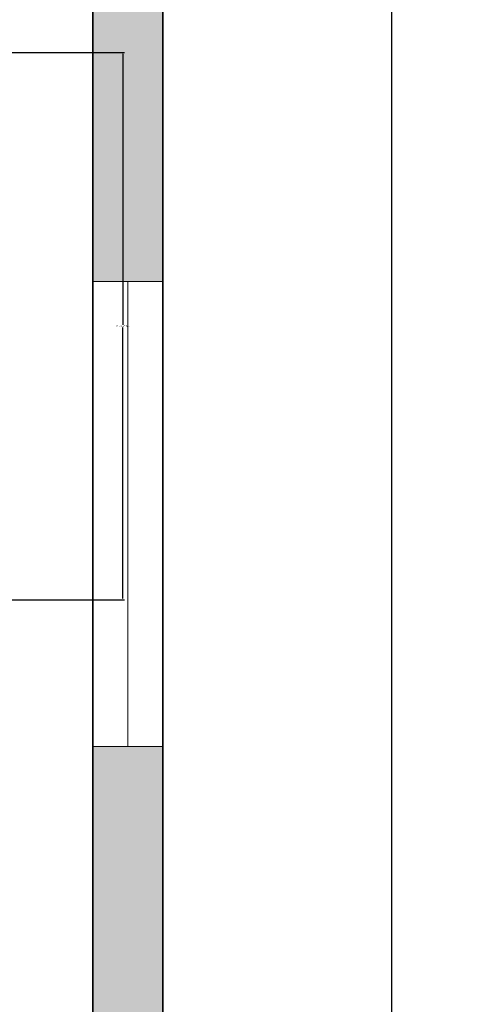
# Model space of a CAD drawing. Units: inches. Extents: x -15 to 423, y -713 to 71.
# Tile 23 of 24: x 364 to 423, y -224 to -97. Entities that reach past the tile are written whole.
import ezdxf

# ---------------------------------------------------------------- set-up
doc = ezdxf.new("R2010")
doc.units = ezdxf.units.IN
doc.header["$MEASUREMENT"] = 0
for name, color, linetype, lineweight in [('A-ANNO-DIMS', 2, 'Continuous', 18), ('A-GLAZ', 5, 'Continuous', 18), ('A-WALL', 7, 'Continuous', 35), ('A-WALL-PATT', 8, 'Continuous', 13)]:
    doc.layers.add(name, color=color, linetype=linetype, lineweight=lineweight)
doc.styles.get("Standard").update_dxf_attribs({"font": 'arial.ttf'})
doc.dimstyles.get("Standard").update_dxf_attribs({"dimtxt": 0.18, "dimasz": 0.18, "dimexe": 0.18, "dimexo": 0.0625, "dimgap": 0.09, "dimtad": 0, "dimtih": 1, "dimtoh": 1, "dimdec": 0, "dimzin": 0, "dimdsep": 46, "dimlunit": 3, "dimtxsty": 'Standard', "dimcen": 0.09, "dimadec": 0, "dimazin": 0, "dimtfac": 1, "dimtdec": 0, "dimtofl": 0, "dimtmove": 0, "dimatfit": 3, "dimfxl": 1, "dimtolj": 1, "dimtzin": 0, "dimarcsym": 0})

# ---------------------------------------------------------------- blocks, each defined once
blk = doc.blocks.new('*D9')
at = {"layer": 'A-ANNO-DIMS', "color": 0, "lineweight": -2, "transparency": 16777216}
for p, q in [((382.14, 17.5), (411.79, 17.5)), ((411.61, 17.32), (411.61, -324.61)), ((411.61, -672.82), (411.61, -330.89)), ((382.14, -673), (411.79, -673))]:
    blk.add_line(p, q, dxfattribs=at)
at = {"layer": 'A-ANNO-DIMS', "color": 0, "transparency": 16777216}
for points in [[(411.58, 17.32), (411.64, 17.32), (411.61, 17.5)], [(411.58, -672.82), (411.64, -672.82), (411.61, -673)]]:
    blk.add_solid(points, dxfattribs=at)
at = {"layer": 'Defpoints', "color": 0, "transparency": 16777216}
for p in [(382.08, 17.5), (382.08, -673), (411.61, -673)]:
    blk.add_point(p, dxfattribs=at)
at = {"layer": 'A-ANNO-DIMS', "color": 0, "transparency": 16777216, "insert": (411.61, -327.75), "char_height": 6, "attachment_point": 5}
blk.add_mtext('\\A1;57\'-7"', dxfattribs=at)
blk = doc.blocks.new('WINDOW-60IN')
for p, q in [((0, 9), (60, 9)), ((0, 0), (0, 9)), ((60, 9), (60, 0)), ((0, 4.5), (60, 4.5)), ((60, 0), (0, 0))]:
    blk.add_line(p, q)
blk = doc.blocks.new('*D32')
at = {"layer": 'A-ANNO-DIMS', "color": 0, "lineweight": -2, "transparency": 16777216}
for p, q in [((361.97, -101.28), (377.13, -101.28)), ((376.95, -101.46), (376.95, -136.42)), ((376.95, -171.75), (376.95, -136.79)), ((361.97, -171.93), (377.13, -171.93))]:
    blk.add_line(p, q, dxfattribs=at)
at = {"layer": 'A-ANNO-DIMS', "color": 0, "transparency": 16777216}
for points in [[(376.92, -101.46), (376.98, -101.46), (376.95, -101.28)], [(376.92, -171.75), (376.98, -171.75), (376.95, -171.93)]]:
    blk.add_solid(points, dxfattribs=at)
at = {"layer": 'Defpoints', "color": 0, "transparency": 16777216}
for p in [(361.91, -101.28), (376.95, -101.28), (361.91, -171.93)]:
    blk.add_point(p, dxfattribs=at)
at = {"layer": 'A-ANNO-DIMS', "color": 0, "transparency": 16777216, "insert": (376.95, -136.61), "char_height": 0.18, "attachment_point": 5}
blk.add_mtext('\\A1;5\'-10 1/2" TYP.', dxfattribs=at)

msp = doc.modelspace()

# ---------------------------------------------------------------- hatches: boundary and pattern name
at = {"layer": 'A-WALL-PATT'}
h = msp.add_hatch(color=256, dxfattribs=at)
h.dxf.hatch_style = 1
h.paths.add_polyline_path([(34.08, -349.58), (25.08, -349.58), (25.08, -431), (34.08, -431)])
h.paths.add_polyline_path([(34.08, -467), (25.08, -467), (25.08, -673), (34.08, -673)])
h.paths.add_polyline_path([(373.08, -668.5), (182.08, -668.5), (182.08, -673), (373.08, -673)])
h.paths.add_polyline_path([(253.2, -597.5), (191.08, -597.5), (191.08, -594.5), (182.08, -594.5), (182.08, -606.5), (253.2, -606.5)])
h.paths.add_polyline_path([(373.08, -597.5), (313.2, -597.5), (313.2, -606.5), (373.08, -606.5)])
h.paths.add_polyline_path([(382.08, -545.55), (373.08, -545.55), (373.08, -673), (382.08, -673)])
h.paths.add_polyline_path([(139.08, -488), (34.08, -488), (34.08, -497), (139.08, -497), (139.08, -492.5)])
h.paths.add_polyline_path([(139.08, -396.5), (128.58, -396.5), (128.58, -352.79), (124.08, -352.79), (124.08, -396.5), (34.08, -396.5), (34.08, -410), (139.08, -410), (139.08, -403.25)])
h.paths.add_polyline_path([(191.08, -396.5), (179.08, -396.5), (179.08, -410), (182.08, -410), (182.08, -488), (179.08, -488), (179.08, -497), (182.08, -497), (182.08, -501.43), (191.08, -501.43)])
h.paths.add_polyline_path([(373.08, -396.5), (253.08, -396.5), (253.08, -393.5), (248.58, -393.5), (248.58, -401), (284.58, -401), (284.58, -404), (289.08, -404), (289.08, -401), (373.08, -401)])
h.paths.add_polyline_path([(373.08, -449), (289.08, -449), (289.08, -432), (286.83, -432), (284.58, -432), (284.58, -453.5), (373.08, -453.5)])
h.paths.add_polyline_path([(382.08, -344.27), (373.08, -344.27), (373.08, -413.68), (382.08, -413.68)])
h.paths.add_polyline_path([(382.08, -437.68), (373.08, -437.68), (373.08, -485.55), (382.08, -485.55)])
h.paths.add_polyline_path([(34.08, -188.26), (25.08, -188.26), (25.08, -289.58), (34.08, -289.58)])
h.paths.add_polyline_path([(164.08, -236), (34.08, -236), (34.08, -240.5), (124.08, -240.5), (124.08, -293.12), (128.58, -293.12), (128.58, -240.5), (164.08, -240.5), (164.08, -238.25)])
h.paths.add_polyline_path([(373.08, -236), (242.58, -236), (242.58, -238.25), (242.58, -240.5), (248.58, -240.5), (248.58, -353.5), (250.83, -353.5), (253.08, -353.5), (253.08, -240.5), (373.08, -240.5)])
h.paths.add_polyline_path([(382.08, -190.86), (373.08, -190.86), (373.08, -284.27), (382.08, -284.27)])
h.paths.add_polyline_path([(211.58, -80), (253.58, -80), (253.58, -77.75), (253.58, -75.5), (153.58, -75.5), (153.58, -77.75), (153.58, -80), (207.08, -80), (207.08, -236), (204.08, -236), (204.08, -240.5), (214.58, -240.5), (214.58, -236), (211.58, -236)])
h.paths.add_polyline_path([(34.08, 8.5), (70.36, 8.5), (70.36, 17.5), (25.08, 17.5), (25.08, -128.26), (34.08, -128.26)])
h.paths.add_polyline_path([(110.58, 17.5), (94.36, 17.5), (94.36, 8.5), (110.58, 8.5)])
h.paths.add_polyline_path([(296.58, 17.5), (110.58, 17.5), (110.58, 13), (296.58, 13)])
h.paths.add_polyline_path([(110.58, 8.5), (106.08, 8.5), (106.08, -75.5), (103.08, -75.5), (103.08, -80), (113.58, -80), (113.58, -77.75), (113.58, -75.5), (110.58, -75.5)])
h.paths.add_polyline_path([(75.08, -75.5), (34.08, -75.5), (34.08, -80), (75.08, -80), (75.08, -77.75)])
h.paths.add_polyline_path([(343.09, 17.5), (296.58, 17.5), (296.58, 13), (296.58, 8.5), (343.09, 8.5)])
h.paths.add_polyline_path([(304.08, -75.5), (301.08, -75.5), (301.08, 8.5), (296.58, 8.5), (296.58, -75.5), (293.58, -75.5), (293.58, -80), (304.08, -80)])
h.paths.add_polyline_path([(382.08, 17.5), (367.09, 17.5), (367.09, 8.5), (373.08, 8.5), (373.08, -130.86), (382.08, -130.86)])
h.paths.add_polyline_path([(373.08, -75.5), (332.08, -75.5), (332.08, -77.75), (332.08, -80), (373.08, -80)])

# ---------------------------------------------------------------- linework, layer by layer
at = {"layer": 'A-WALL'}
for p, q in [((382.08, 17.5), (382.08, -673)), ((373.08, 8.5), (373.08, -673))]:
    msp.add_line(p, q, dxfattribs=at)

# ---------------------------------------------------------------- block references
at = {"layer": 'A-GLAZ', "rotation": 90.00000000000011}
msp.add_blockref('WINDOW-60IN', (382.08, -190.86), dxfattribs=at)

# ---------------------------------------------------------------- dimensions: what is measured, and where the dimension line sits
at = {"layer": 'A-ANNO-DIMS'}
dim = msp.add_linear_dim(base=(411.6050599, -672.99989936), p1=(382.08055573, 17.50010064), p2=(382.08055573, -672.99989936), angle=90, dimstyle='Standard', override={"dimtxt": 6, "dimclrd": 0, "dimclre": 0, "dimclrt": 0}, dxfattribs=at)
dim.commit()
dim.dimension.update_dxf_attribs({"geometry": '*D9', "text_midpoint": (411.6050599, -327.74989936)})
dim = msp.add_linear_dim(base=(376.9456, -101.2826), p1=(361.9055, -171.928), p2=(361.9055, -101.2826), angle=90, text='<> TYP.', dimstyle='Standard', override={"dimdec": 1, "dimlfac": 1, "dimrnd": 0, "dimzin": 1, "dimdsep": 46, "dimlunit": 4, "dimfrac": 2}, dxfattribs=at)
dim.commit()
dim.dimension.update_dxf_attribs({"geometry": '*D32', "text_midpoint": (376.9456, -136.6053)})

doc.saveas('drawing.dxf')
